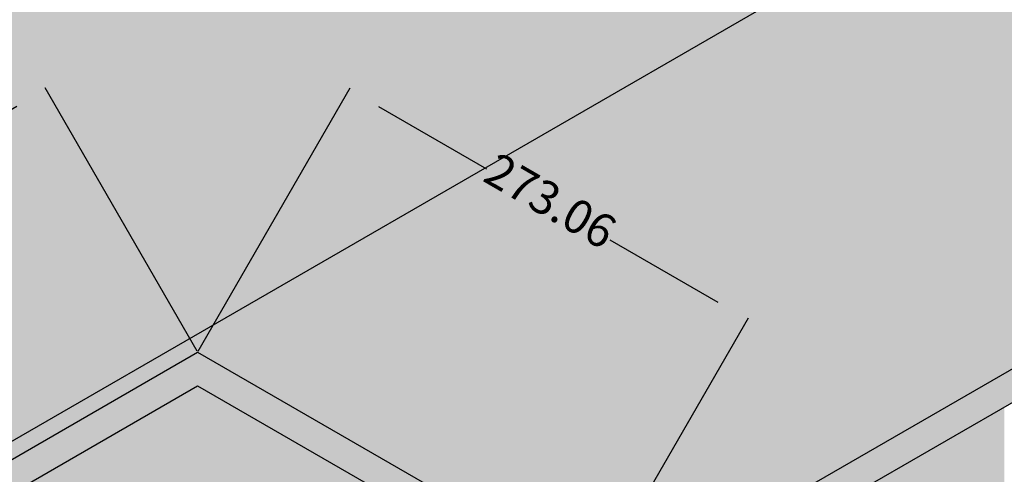
# Model space of a CAD drawing. Units: millimetres. Extents: x 78378 to 86415, y 148682 to 152721.
# Tile 5 of 18: x 79199 to 79783, y 150225 to 150495. Entities that reach past the tile are written whole.
import ezdxf

# ---------------------------------------------------------------- set-up
doc = ezdxf.new("R2010")
doc.units = ezdxf.units.MM
for name, color, linetype, lineweight in [('A-ANNO-DIMS', 2, 'Continuous', 18), ('A-FURN', 4, 'Continuous', 25), ('A-FURN-PATT', 32, 'Continuous', 13)]:
    doc.layers.add(name, color=color, linetype=linetype, lineweight=lineweight)
doc.styles.get("Standard").update_dxf_attribs({"font": 'arial.ttf'})
doc.dimstyles.new('ISO-25', dxfattribs={"dimtxt": 20, "dimasz": 20, "dimexe": 1.25, "dimexo": 0.625, "dimtad": 0, "dimdec": 1, "dimtxsty": 'Standard', "dimcen": 2.5, "dimadec": 0, "dimazin": 0, "dimtfac": 1, "dimtdec": 1, "dimtmove": 0, "dimatfit": 3, "dimfxl": 1, "dimarcsym": 0})

# ---------------------------------------------------------------- blocks, each defined once
blk = doc.blocks.new('*D23')
at = {"layer": 'A-ANNO-DIMS', "color": 0, "lineweight": -2, "transparency": 16777216}
for p, q in [((79304.01, 150298.13), (79213.69, 150454.55)), ((79197, 150443.47), (79082.34, 150377.27)), ((78908.24, 150276.76), (79022.89, 150342.95)), ((78980.6, 150111.41), (78890.29, 150267.84))]:
    blk.add_line(p, q, dxfattribs=at)
at = {"layer": 'A-ANNO-DIMS', "color": 0, "transparency": 16777216}
for points in [[(79195.33, 150446.36), (79198.67, 150440.59), (79214.32, 150453.47)], [(78906.57, 150279.64), (78909.9, 150273.87), (78890.92, 150266.76)]]:
    blk.add_solid(points, dxfattribs=at)
at = {"layer": 'Defpoints', "color": 0, "transparency": 16777216}
for p in [(79214.32, 150453.47), (79304.32, 150297.59), (78980.92, 150110.87)]:
    blk.add_point(p, dxfattribs=at)
at = {"layer": 'A-ANNO-DIMS', "color": 0, "transparency": 16777216, "insert": (79052.62, 150360.11), "char_height": 20, "attachment_point": 5, "rotation": 30}
blk.add_mtext('373.4', dxfattribs=at)
blk = doc.blocks.new('*D24')
at = {"layer": 'A-ANNO-DIMS', "color": 0, "lineweight": -2, "transparency": 16777216}
for p, q in [((79304.63, 150298.13), (79394.94, 150454.55)), ((79411.64, 150443.47), (79475.92, 150406.36)), ((79613.48, 150326.94), (79549.2, 150364.05)), ((79541.11, 150161.6), (79631.43, 150318.02))]:
    blk.add_line(p, q, dxfattribs=at)
at = {"layer": 'A-ANNO-DIMS', "color": 0, "transparency": 16777216}
for points in [[(79413.31, 150446.36), (79409.97, 150440.59), (79394.32, 150453.47)], [(79615.15, 150329.83), (79611.81, 150324.05), (79630.8, 150316.94)]]:
    blk.add_solid(points, dxfattribs=at)
at = {"layer": 'Defpoints', "color": 0, "transparency": 16777216}
for p in [(79630.8, 150316.94), (79304.32, 150297.59), (79540.8, 150161.06)]:
    blk.add_point(p, dxfattribs=at)
at = {"layer": 'A-ANNO-DIMS', "color": 0, "transparency": 16777216, "insert": (79512.56, 150385.21), "char_height": 20, "attachment_point": 5, "rotation": 330}
blk.add_mtext('273.06', dxfattribs=at)

msp = doc.modelspace()

# ---------------------------------------------------------------- hatches: boundary and pattern name
at = {"layer": 'A-FURN-PATT'}
h = msp.add_hatch(color=256, dxfattribs=at)
h.dxf.hatch_style = 1
h.paths.add_polyline_path([(78839.3276, 151040.0076), (78579.52, 151190.0076), (78579.52, 150470.0076), (78839.3276, 150320.0076)])
h.paths.add_polyline_path([(79073.1545, 150899.6469, 0.27777969), (79002.2645, 150996.3205, 0.79108393), (78917.9567, 150978.8719, 0.18044832), (78856.6481, 150853.0138), (78856.6481, 150350.6973), (79073.1545, 150484.318)])
h.paths.add_polyline_path([(79073.1545, 151175.0076), (78856.6481, 151050.0076), (78856.6481, 150853.0138, -0.18044832), (78917.9567, 150978.8719, -0.79108393), (79002.2645, 150996.3205, -0.27777969), (79073.1545, 150899.6469)])
h.paths.add_polyline_path([(79341.6224, 151350.0076), (79099.1352, 151490.0076), (78596.8405, 151200.0076), (78839.3276, 151060.0076)])
h.paths.add_polyline_path([(79904.5389, 151675.0076), (79662.0518, 151815.0076), (79099.1352, 151490.0076), (79341.6224, 151350.0076)])
h.paths.add_polyline_path([(80389.5131, 151955.0076), (80389.5131, 152235.0076), (79662.0518, 151815.0076), (79904.5389, 151675.0076)])
h.paths.add_polyline_path([(80389.5131, 151955.0076), (80164.3465, 151825.0076), (80164.3465, 151105.0076), (80614.6797, 151105.0076), (80614.6797, 151825.0076)])
edge = h.paths.add_edge_path(flags=16)
edge.add_spline(control_points=[(80216.308, 151728.251), (80227.1854, 151732.981), (80256.3301, 151745.6544), (80298.41, 151761.9595), (80340.2597, 151805.855), (80391.0771, 151782.0404), (80454.0396, 151805.7581), (80496.5007, 151742.4095), (80543.8218, 151733.4043), (80562.7182, 151729.8083)], knot_values=[0, 0, 0, 0, 35.54374676, 95.23575347, 136.36767513, 200.93298197, 236.72641081, 322.88993498, 380.17027367, 380.17027367, 380.17027367, 380.17027367], degree=3, periodic=0)
edge.add_line((80562.7182, 151729.8083), (80562.7182, 151165.0076))
edge.add_line((80562.7182, 151165.0076), (80216.308, 151165.0076))
edge.add_line((80216.308, 151165.0076), (80216.308, 151728.251))
h.paths.add_polyline_path([(80632.0002, 152095.0076), (80389.5131, 152235.0076), (80389.5131, 151955.0076), (80614.6797, 151825.0076), (80632.0002, 151815.0076)])
h.paths.add_polyline_path([(80867.7794, 151958.8805), (80632.0002, 152095.0076), (80632.0002, 151815.0076), (80632.0002, 151510.0076), (80867.7794, 151373.8805)])
h.paths.add_polyline_path([(80147.026, 151495.8203, 0.18918979), (80063.5671, 151597.7244, 0.78826136), (79979.2691, 151580.5832, 0.16072613), (79904.5389, 151413.5769), (79904.5389, 150955.0076), (80147.026, 151095.0076)])
h.paths.add_polyline_path([(80147.026, 151815.0076), (79904.5389, 151675.0076), (79904.5389, 151413.5769, -0.16072613), (79979.2691, 151580.5832, -0.78826136), (80063.5671, 151597.7244, -0.18918979), (80147.026, 151495.8203)])
h.paths.add_polyline_path([(79887.2184, 151645.0076), (79640.4011, 151502.5076), (79640.4011, 151262.3325, -0.16072613), (79715.1313, 151429.3387, -0.78826136), (79799.4294, 151446.48, -0.21290578), (79887.2184, 151328.7247)])
h.paths.add_polyline_path([(79799.4294, 151446.48, 0.78826136), (79715.1313, 151429.3387, 0.16072613), (79640.4011, 151262.3325), (79640.4011, 150822.5076), (79887.2184, 150965.0076), (79887.2184, 151328.7247, 0.21290578)])
h.paths.add_polyline_path([(79605.7601, 151482.5076), (79358.9429, 151340.0076), (79358.9429, 151100.0701, -0.16072613), (79433.6731, 151267.0764, -0.78826136), (79517.9711, 151284.2176, -0.21290578), (79605.7601, 151166.4623)])
h.paths.add_polyline_path([(79605.7601, 151166.4623, 0.21290578), (79517.9711, 151284.2176, 0.78826136), (79433.6731, 151267.0764, 0.16072613), (79358.9429, 151100.0701), (79358.9429, 150742.9831), (79419.0877, 150694.7323), (79605.7601, 150802.5076)])
edge = h.paths.add_edge_path(flags=0)
edge.add_spline(control_points=[(81152.4356, 151098.7676), (81105.7208, 151145.9466), (81038.6136, 151213.7208), (80882.3866, 151214.1938), (80797.4434, 151311.2997), (80711.8686, 151340.3754), (80681.7691, 151350.6023)], knot_values=[0, 0, 0, 0, 188.233441, 270.4032752, 445.45179201, 540.42858829, 540.42858829, 540.42858829, 540.42858829], degree=3, periodic=0)
edge.add_line((80683.4538, 151350.0269), (80683.4538, 151104.8792))
edge.add_line((80683.4538, 151104.8792), (81152.4356, 150851.399))
edge.add_line((81152.4356, 150851.399), (81152.4356, 151098.7676))
edge = h.paths.add_edge_path(flags=0)
edge.add_spline(control_points=[(80912.9018, 151027.1103), (80892.3742, 151034.1027), (80860.1663, 151045.0739), (80835.5097, 151068.1214), (80826.5679, 151076.4797)], knot_values=[0, 0, 0, 0, 63.98405104, 100.39142428, 100.39142428, 100.39142428, 100.39142428], degree=3, periodic=0)
edge.add_arc((80830.0414, 151081.2992), 5.9407, 100.9277276, 234.2187381, ccw=False)
edge.add_spline(control_points=[(80828.9152, 151087.1322), (80837.857, 151078.7739), (80862.5136, 151055.7263), (80894.7215, 151044.7552), (80915.2491, 151037.7628)], knot_values=[0, 0, 0, 0, 36.40737324, 100.39142428, 100.39142428, 100.39142428, 100.39142428], degree=3, periodic=0)
edge.add_arc((80914.7882, 151032.2795), 5.5026, -107.9540399, 85.195579, ccw=False)
h.paths.add_polyline_path([(81238.218, 151110.0076), (80632.0002, 151460.0076), (80632.0002, 151105.0076), (81238.218, 150755.0076)])
edge = h.paths.add_edge_path(flags=16)
edge.add_line((81152.4356, 150851.399), (80683.4538, 151104.8792))
edge.add_line((80683.4538, 151104.8792), (80683.4538, 151350.0279))
edge.add_spline(control_points=[(80681.7691, 151350.6023), (80711.8686, 151340.3754), (80797.4434, 151311.2997), (80882.3866, 151214.1938), (81038.6136, 151213.7208), (81105.7208, 151145.9466), (81152.4356, 151098.7676)], knot_values=[0, 0, 0, 0, 94.97679628, 270.02531309, 352.19514729, 540.42858829, 540.42858829, 540.42858829, 540.42858829], degree=3, periodic=0)
edge.add_line((81152.4356, 151098.7676), (81152.4356, 150851.399))
edge = h.paths.add_edge_path(flags=0)
edge.add_spline(control_points=[(80912.9018, 151027.1103), (80892.3742, 151034.1027), (80860.1663, 151045.0739), (80835.5097, 151068.1214), (80826.5679, 151076.4797)], knot_values=[0, 0, 0, 0, 63.98405104, 100.39142428, 100.39142428, 100.39142428, 100.39142428], degree=3, periodic=0)
edge.add_arc((80830.0414, 151081.2992), 5.9407, 100.9277276, 234.2187381, ccw=False)
edge.add_spline(control_points=[(80828.9152, 151087.1322), (80837.857, 151078.7739), (80862.5136, 151055.7263), (80894.7215, 151044.7552), (80915.2491, 151037.7628)], knot_values=[0, 0, 0, 0, 36.40737324, 100.39142428, 100.39142428, 100.39142428, 100.39142428], degree=3, periodic=0)
edge.add_arc((80914.7882, 151032.2795), 5.5026, -107.7417882, 85.195579, ccw=False)
h.paths.add_polyline_path([(81498.0256, 151255.0076), (81238.218, 151110.0076), (81238.218, 150755.0076), (81498.0256, 150905.0076)])
edge = h.paths.add_edge_path(flags=16)
edge.add_spline(control_points=[(81152.4356, 151098.7676), (81105.7208, 151145.9466), (81038.6136, 151213.7208), (80882.3866, 151214.1938), (80797.4434, 151311.2997), (80711.8686, 151340.3754), (80681.7691, 151350.6023)], knot_values=[0, 0, 0, 0, 188.233441, 270.4032752, 445.45179201, 540.42858829, 540.42858829, 540.42858829, 540.42858829], degree=3, periodic=0)
edge.add_line((80683.4538, 151350.0279), (80683.4538, 151104.8792))
edge.add_line((80683.4538, 151104.8792), (81152.4356, 150851.399))
edge.add_line((81152.4356, 150851.399), (81152.4356, 151098.7676))
h.paths.add_polyline_path([(81453.9904, 151280.4314), (80867.7794, 151618.8805), (80867.7794, 151373.8805), (81238.218, 151160.0076)])
edge = h.paths.add_edge_path(flags=16)
edge.add_line((81189.2304, 151297.6373), (81114.4166, 151300.2154))
edge.add_arc((81412.0967, 151394.0167), 312.1092, 179.7569303, 197.4900342, ccw=False)
edge.add_ellipse((81154.0183, 151392.0436), major_axis=(-54.0264, 3.6301), ratio=0.22179693, start_angle=0, end_angle=0.3517985, ccw=False)
edge.add_ellipse((81154.0183, 151392.0436), major_axis=(-54.0264, 3.6301), ratio=0.22179693, start_angle=180, end_angle=360, ccw=False)
edge.add_spline(control_points=[(81196.1844, 151321.9476), (81224.9802, 151347.1455), (81266.8846, 151383.8144), (81222.0354, 151387.0304), (81208.0056, 151388.0364)], knot_values=[0, 0, 0, 0, 75.09175173, 109.27580439, 109.27580439, 109.27580439, 109.27580439], degree=3, periodic=0)
edge.add_arc((80751.9112, 151435.6145), 458.5693, 342.4891602, 345.646172, ccw=False)
edge = h.paths.add_edge_path(flags=0)
edge.add_spline(control_points=[(81196.6193, 151323.657), (81197.893, 151324.7717), (81199.1654, 151325.8858), (81209.0233, 151334.5343), (81217.3959, 151341.9835), (81228.0928, 151352.5012), (81231.3883, 151355.9524), (81236.9493, 151362.4395), (81239.214, 151365.4773), (81241.4987, 151369.416), (81242.064, 151370.5542), (81242.9187, 151372.6971), (81243.2076, 151373.7015), (81243.5012, 151375.5539), (81243.5065, 151376.4), (81243.2432, 151377.9407), (81242.9775, 151378.6373), (81242.1402, 151379.937), (81241.5659, 151380.5416), (81240.2039, 151381.533), (81239.4963, 151381.9384), (81237.0619, 151383.0663), (81235.0242, 151383.6999), (81230.352, 151384.7569), (81227.7173, 151385.1826), (81221.9118, 151385.9145), (81218.7193, 151386.2133), (81213.7912, 151386.6115), (81212.1252, 151386.7359), (81209.6196, 151386.9181), (81208.7865, 151386.9779), (81207.9009, 151387.0432)], knot_values=[0.01548744, 0.01548744, 0.01548744, 0.01548744, 3.33787957, 3.33787957, 25.85130624, 25.85130624, 37.52811308, 37.52811308, 49.20491992, 49.20491992, 54.2850938, 54.2850938, 59.36526768, 59.36526768, 64.44544157, 64.44544157, 69.52561545, 69.52561545, 74.60578933, 74.60578933, 78.49366785, 78.49366785, 86.25567095, 86.25567095, 94.01767406, 94.01767406, 102.20226556, 102.20226556, 106.29456131, 106.29456131, 108.32522175, 108.32522175, 108.32522175, 108.32522175], degree=3, periodic=0)
edge = h.paths.add_edge_path(flags=16)
edge.add_arc((81034.1732, 151350.4693), 42.5822, 231.2679035, 306.151846, ccw=False)
edge.add_line((81007.5303, 151317.2517), (81007.5303, 151395.181))
edge.add_ellipse((81033.412, 151394.7791), major_axis=(-25.8816, 0.4538), ratio=0.23894509, start_angle=0, end_angle=0.1147075, ccw=False)
edge.add_ellipse((81033.412, 151394.7791), major_axis=(-25.8816, 0.4538), ratio=0.23894509, start_angle=181.1677709, end_angle=358.9476457, ccw=False)
edge.add_ellipse((81033.412, 151395.7791), major_axis=(-25.8816, 0.4538), ratio=0.23894509, start_angle=180, end_angle=360.1147075, ccw=False)
edge.add_ellipse((81033.412, 151395.7791), major_axis=(-25.8816, 0.4538), ratio=0.23894509, start_angle=178.9476457, end_angle=180, ccw=False)
edge.add_line((81059.2936, 151395.1778), (81059.2936, 151394.3772))
edge.add_ellipse((81033.412, 151394.7791), major_axis=(-25.8816, 0.4538), ratio=0.23894509, start_angle=180, end_angle=180.1147075, ccw=False)
edge.add_ellipse((81033.412, 151394.7791), major_axis=(-25.8816, 0.4538), ratio=0.23894509, start_angle=3.6903098, end_angle=176.4406503, ccw=False)
edge.add_line((81059.2936, 151393.3388), (81059.2936, 151316.086))
h.paths.add_polyline_path([(80951.9355, 151343.9568), (80909.6838, 151362.4635), (80904.0219, 151443.9615, -0.38133308), (80987.2169, 151411.3717)], flags=16)
h = msp.add_hatch(color=256, dxfattribs=at)
h.dxf.hatch_style = 1
h.paths.add_polyline_path([(80389.8136, 150935.1811), (80389.5131, 151105.0076), (80164.3465, 151105.0076), (79904.5389, 150955.0076), (79433.5848, 150683.1022), (79459.4128, 150662.3818), (79243.9048, 150537.9582), (79160.4069, 150518.1674), (78839.3276, 150320.0076), (78579.52, 150470.0076), (78570.8597, 150475.0076), (78570.8597, 150465.0076), (78570.8597, 149885.0076)])
h.paths.add_polyline_path([(80086.4042, 150460.0076), (79826.5966, 150610.0076), (78570.8597, 149885.0076), (78830.6674, 149735.0076)])
h.paths.add_polyline_path([(79540.8001, 150161.0557), (79217.3967, 149974.3386), (78980.9166, 150110.8705), (79304.32, 150297.5875)], flags=16)
h.paths.add_polyline_path([(79506.159, 150161.0557), (79217.3967, 149994.3386), (79015.5576, 150110.8705), (79304.32, 150277.5875)], flags=0)
edge = h.paths.add_edge_path(flags=0)
edge.add_arc((79247.8636, 150177.1541), 137.9799, 256.0025928, 293.5594109)
edge.add_arc((79240.7671, 150078.2605), 68.0855, 336.099104, 387.3696877)
edge.add_ellipse((79258.3074, 150109.4852), major_axis=(-42.6234, -1.6591), ratio=0.16042843, start_angle=0, end_angle=179.0977279, ccw=False)
edge.add_arc((79285.2112, 150074.2509), 77.2096, 155.1233104, 203.6557939)
edge = h.paths.add_edge_path(flags=0)
edge.add_ellipse((79258.6958, 150110.8297), major_axis=(-42.6234, -1.6591), ratio=0.16042843, start_angle=350.6039412, end_angle=356.2289762)
edge.add_line((79219.169, 150111.8937), (79218.3268, 150109.4141))
edge.add_arc((79262.4675, 150032.9602), 88.2813, 112.3931229, 120, ccw=False)
h.paths.add_polyline_path([(79287.0625, 150086.9703, -0.24770206), (79288.1967, 150077.2955, -0.39047651), (79265.4731, 150072.5438, -0.48726153), (79264.079, 150082.3769, 0.39560433)], flags=0)
h.paths.add_polyline_path([(80389.5131, 150935.0076), (79826.5966, 150610.0076), (80086.4042, 150460.0076), (80692.622, 150460.0076), (80952.4296, 150610.0076)])
edge = h.paths.add_edge_path(flags=16)
edge.add_ellipse((80392.4466, 150825.601), major_axis=(-133.0757, 7.722), ratio=0.42449957, start_angle=0, end_angle=360)
edge = h.paths.add_edge_path(flags=0)
edge.add_spline(control_points=[(80269.3541, 150832.7436), (80269.2919, 150831.672), (80269.3503, 150830.5922), (80269.7341, 150828.3361), (80270.0612, 150827.1587), (80271.0461, 150824.6748), (80271.7052, 150823.3692), (80273.4061, 150820.6503), (80274.4481, 150819.2381), (80276.9366, 150816.3509), (80278.3828, 150814.8762), (80282.5858, 150811.0913), (80285.6261, 150808.7701), (80292.6031, 150804.2267), (80296.5388, 150802.0041), (80305.195, 150797.7581), (80309.9151, 150795.7344), (80320.0112, 150791.96), (80325.387, 150790.2092), (80339.2162, 150786.315), (80347.9578, 150784.3563), (80366.0679, 150781.2568), (80375.4359, 150780.1158), (80394.3093, 150778.7158), (80403.8142, 150778.4568), (80422.4656, 150778.8319), (80431.6115, 150779.4662), (80449.0608, 150781.5838), (80457.3636, 150783.0675), (80472.6699, 150786.7766), (80479.6726, 150789.0033), (80490.1894, 150793.2813), (80494.1268, 150795.1967), (80501.0146, 150799.1885), (80503.9632, 150801.2651), (80508.2066, 150804.9015), (80509.73, 150806.4609), (80512.1996, 150809.4942), (80513.1456, 150810.9657), (80514.4291, 150813.5431), (80514.8436, 150814.6688), (80515.3984, 150816.8625), (80515.5405, 150817.9315), (80515.5801, 150820.098), (80515.4773, 150821.1978), (80514.9905, 150823.5062), (80514.6047, 150824.7154), (80513.4854, 150827.2641), (80512.7511, 150828.6027), (80510.8872, 150831.3809), (80509.7578, 150832.8196), (80507.0873, 150835.7513), (80505.5466, 150837.2439), (80501.0624, 150841.0944), (80497.8199, 150843.4576), (80490.4174, 150848.062), (80486.2582, 150850.3037), (80477.1448, 150854.5643), (80472.1909, 150856.5835), (80461.6275, 150860.3245), (80456.0182, 150862.0465), (80441.7332, 150865.8127), (80432.7885, 150867.6675), (80414.3391, 150870.5317), (80404.8349, 150871.5411), (80385.7707, 150872.6572), (80376.2113, 150872.764), (80357.5444, 150872.0728), (80348.4375, 150871.2748), (80331.1682, 150868.83), (80323.0064, 150867.1827), (80309.472, 150863.5363), (80303.8628, 150861.6593), (80293.8018, 150857.5401), (80289.3512, 150855.2969), (80282.7757, 150851.2345), (80280.3473, 150849.4579), (80276.2606, 150845.9127), (80274.604, 150844.1458), (80272.3157, 150841.1243), (80271.5358, 150839.8454), (80270.3496, 150837.3879), (80269.9417, 150836.2101), (80269.5065, 150834.2815), (80269.3988, 150833.5143), (80269.3541, 150832.7436)], knot_values=[0, 0, 0, 0, 0.09750046, 0.09750046, 0.19500092, 0.19500092, 0.29250138, 0.29250138, 0.39000184, 0.39000184, 0.4875023, 0.4875023, 0.63880322, 0.63880322, 0.79010415, 0.79010415, 0.94140507, 0.94140507, 1.092706, 1.092706, 1.3128171, 1.3128171, 1.5329282, 1.5329282, 1.7530393, 1.7530393, 1.97315041, 1.97315041, 2.19326151, 2.19326151, 2.41337261, 2.41337261, 2.56986063, 2.56986063, 2.72634866, 2.72634866, 2.84418658, 2.84418658, 2.96202451, 2.96202451, 3.06023388, 3.06023388, 3.15844325, 3.15844325, 3.25665261, 3.25665261, 3.35486198, 3.35486198, 3.45307135, 3.45307135, 3.55128072, 3.55128072, 3.64949009, 3.64949009, 3.80392773, 3.80392773, 3.95836537, 3.95836537, 4.11280301, 4.11280301, 4.26724064, 4.26724064, 4.48920349, 4.48920349, 4.71116635, 4.71116635, 4.9331292, 4.9331292, 5.15509205, 5.15509205, 5.3770549, 5.3770549, 5.55785361, 5.55785361, 5.73865232, 5.73865232, 5.87239556, 5.87239556, 6.00613879, 6.00613879, 6.109605, 6.109605, 6.2130712, 6.2130712, 6.28318531, 6.28318531, 6.28318531, 6.28318531], degree=3, periodic=0)
edge = h.paths.add_edge_path(flags=0)
edge.add_ellipse((80392.4466, 150825.601), major_axis=(-101.8398, 3.3923), ratio=0.40349248, start_angle=0, end_angle=360)
edge = h.paths.add_edge_path(flags=0)
edge.add_ellipse((80391.1657, 150858.3746), major_axis=(9.0882, -0.6733), ratio=0.35135413, start_angle=0, end_angle=360)
h.paths.add_polyline_path([(80952.4296, 150610.0076), (80692.622, 150460.0076), (81361.2342, 150073.9842), (81649.9628, 150052.7286), (81766.4935, 150120.0076), (81766.4935, 150140.0076), (81564.9025, 150256.3963), (81564.8884, 150096.1963), (81538.9076, 150111.1963), (81538.9217, 150271.3963)])
h.paths.add_polyline_path([(81539.0357, 151571.3305), (80867.7794, 151958.8805), (80867.7794, 151618.8805), (81498.0256, 151255.0076), (81498.0256, 150905.0076), (81238.218, 150755.0076), (81538.9488, 150581.3806)])
h.paths.add_polyline_path([(81766.4935, 151440.0076), (81565.0164, 151556.3305), (81564.9296, 150566.3806), (81766.4935, 150450.0076)])
edge = h.paths.add_edge_path()
edge.add_line((81564.9296, 150566.3806), (81564.9137, 150384.6289))
edge.add_ellipse((81552.1304, 150358.5718), major_axis=(52.6272, 3.506), ratio=0.49589905, start_angle=367.5169757, end_angle=420.0564686, ccw=False)
edge.add_ellipse((81552.1304, 150358.5718), major_axis=(52.6272, 3.506), ratio=0.49589905, start_angle=351.729742, end_angle=367.5169757, ccw=False)
edge.add_ellipse((81552.1304, 150345.5016), major_axis=(52.6272, 3.506), ratio=0.49589905, start_angle=352.5116949, end_angle=366.3006092, ccw=False)
edge.add_line((81603.4463, 150342.2039), (81603.5064, 150340.4475))
edge.add_ellipse((81552.1304, 150332.128), major_axis=(52.6272, 3.506), ratio=0.49589905, start_angle=353.6729654, end_angle=365.3867997, ccw=False)
edge.add_ellipse((81552.1304, 150332.128), major_axis=(52.6272, 3.506), ratio=0.49589905, start_angle=350.9388331, end_angle=353.6729654)
edge.add_line((81603.8688, 150329.855), (81604.0442, 150324.7302))
edge.add_ellipse((81552.1304, 150317.7418), major_axis=(52.6272, 3.506), ratio=0.49589905, start_angle=355.2176746, end_angle=363.8553364, ccw=False)
edge.add_ellipse((81552.1304, 150317.7418), major_axis=(52.6272, 3.506), ratio=0.49589905, start_angle=341.3250873, end_angle=355.2176746, ccw=False)
edge.add_ellipse((81552.1304, 150317.7418), major_axis=(52.6272, 3.506), ratio=0.49589905, start_angle=293.4661701, end_angle=341.3250873, ccw=False)
edge.add_line((81564.9057, 150292.9664), (81564.9025, 150256.3963))
edge.add_line((81564.9025, 150256.3963), (81766.4935, 150140.0076))
edge.add_line((81766.4935, 150140.0076), (81766.4935, 150450.0076))
edge.add_line((81766.4935, 150450.0076), (81564.9296, 150566.3806))
h.paths.add_polyline_path([(81525.5713, 150321.598), (81526.5985, 150321.3069), (81528.6771, 150320.947)])
h.paths.add_polyline_path([(81512.7903, 150326.1129), (81514.5058, 150325.3887), (81512.538, 150326.2678)])
h.paths.add_polyline_path([(81533.2148, 150320.1615), (81534.6952, 150319.9052), (81536.5995, 150319.7557)])
h.paths.add_polyline_path([(81518.622, 150323.6513), (81519.227, 150323.3959), (81521.289, 150322.8116)])
h.paths.add_polyline_path([(81501.2183, 150336.2599), (81500.3543, 150338.1339), (81499.7815, 150340.0494), (81499.5032, 150341.9955), (81499.5032, 150343.7257), (81499.7584, 150345.5905), (81500.2766, 150347.4549), (81501.0551, 150349.3095), (81501.0967, 150349.3937), (81501.1389, 150349.4778), (81500.9978, 150349.7496), (81500.8628, 150350.0225), (81499.5032, 150355.0658), (81499.9591, 150359.5002), (81501.8982, 150363.9083), (81505.2653, 150368.1646), (81509.9647, 150372.1482), (81515.8627, 150375.7459), (81522.7918, 150378.8553), (81530.555, 150381.3882), (81538.9315, 150383.2724), (81538.9488, 150581.3806), (80632.0002, 151105.0076), (80389.5131, 151105.0076), (80389.8142, 150934.8338), (80952.4296, 150610.0076), (81538.9217, 150271.3963), (81538.9234, 150291.7194), (81538.8752, 150291.721), (81530.1915, 150292.8239), (81522.1802, 150294.6904), (81515.0866, 150297.2633), (81509.8635, 150299.9959), (81505.6084, 150303.1351), (81502.419, 150306.6088), (81500.3683, 150310.3375), (81499.5032, 150314.2358), (81499.5032, 150315.9659), (81499.8206, 150318.1159), (81500.487, 150320.2634), (81501.4979, 150322.3941), (81500.487, 150324.4233), (81499.8206, 150326.5039), (81499.5032, 150328.622), (81499.5032, 150330.3521), (81499.7815, 150332.3262), (81500.3543, 150334.2992)])
h = msp.add_hatch(color=256, dxfattribs=at)
h.dxf.hatch_style = 1
h.paths.add_polyline_path([(79090.475, 151205.0076), (78839.3276, 151060.0076), (78839.3276, 150320.0076), (79090.475, 150475.0076)])
h.paths.add_polyline_path([(79073.1545, 151175.0076), (79073.1545, 150899.6469, -0.04544363), (79073.1545, 150878.5653), (79073.1545, 150484.318), (78856.6481, 150350.6973), (78856.6481, 150814.5249, -0.04815716), (78856.6481, 150853.0138), (78856.6481, 151050.0076)], flags=16)
h.paths.add_polyline_path([(79358.9429, 151340.0076), (79605.7601, 151482.5076), (79605.7601, 150802.5076), (79419.0877, 150694.7323), (79433.5848, 150683.1022), (79623.0806, 150792.5076), (79623.0806, 151512.5076), (79341.6224, 151350.0076), (79341.6224, 150756.8784), (79358.9429, 150742.9831)])
h.paths.add_polyline_path([(79341.6224, 151350.0076), (79090.475, 151205.0076), (79090.475, 150475.0076), (79160.4069, 150518.1674), (79107.7955, 150505.6973), (79107.7955, 151195.0076), (79109.5275, 151196.0076), (79324.3018, 151320.0076), (79324.3018, 150770.7736), (79341.6224, 150756.8784)])
h.paths.add_polyline_path([(79887.2184, 151645.0076), (79887.2184, 151665.0076), (79623.0806, 151512.5076), (79623.0806, 150792.5076), (79887.2184, 150945.0076), (79887.2184, 150965.0076), (79640.4011, 150822.5076), (79640.4011, 151502.5076)])
h.paths.add_polyline_path([(79904.5389, 151655.0076), (79887.2184, 151645.0076), (79887.2184, 150965.0076), (79904.5389, 150975.0076)])
h.paths.add_polyline_path([(80164.3465, 151825.0076), (80147.026, 151815.0076), (80147.026, 151095.0076), (80164.3465, 151105.0076)])
h.paths.add_polyline_path([(80632.0002, 151510.0076), (80632.0002, 151490.0076), (81238.218, 151140.0076), (81471.6045, 151270.2619), (81453.9904, 151280.4314), (81238.218, 151160.0076)])
h.paths.add_polyline_path([(80632.0002, 151490.0076), (80632.0002, 151470.0076), (81238.218, 151120.0076), (81489.2186, 151260.0924), (81471.6045, 151270.2619), (81238.218, 151140.0076)])
h.paths.add_polyline_path([(80632.0002, 151460.0076), (80632.0002, 151105.0076), (81238.218, 150755.0076), (81238.218, 151110.0076)])
edge = h.paths.add_edge_path(flags=16)
edge.add_spline(control_points=[(80681.7691, 151350.6023), (80711.8686, 151340.3754), (80797.4434, 151311.2997), (80882.3866, 151214.1938), (81038.6136, 151213.7208), (81105.7208, 151145.9466), (81152.4356, 151098.7676)], knot_values=[0, 0, 0, 0, 94.97679628, 270.02531309, 352.19514729, 540.42858829, 540.42858829, 540.42858829, 540.42858829], degree=3, periodic=0)
edge.add_line((81152.4356, 151098.7676), (81152.4356, 150851.399))
edge.add_line((81152.4356, 150851.399), (80683.4538, 151104.8792))
edge.add_line((80683.4538, 151104.8792), (80683.4538, 151350.027))
edge = h.paths.add_edge_path(flags=0)
edge.add_spline(control_points=[(80828.9152, 151087.1322), (80837.857, 151078.7739), (80862.5136, 151055.7263), (80894.7215, 151044.7552), (80915.2491, 151037.7628)], knot_values=[0, 0, 0, 0, 36.40737324, 100.39142428, 100.39142428, 100.39142428, 100.39142428], degree=3, periodic=0)
edge.add_arc((80914.7882, 151032.2795), 5.5026, -107.9540399, 85.195579, ccw=False)
edge.add_spline(control_points=[(80912.9018, 151027.1103), (80892.3742, 151034.1027), (80860.1663, 151045.0739), (80835.5097, 151068.1214), (80826.5679, 151076.4797)], knot_values=[0, 0, 0, 0, 63.98405104, 100.39142428, 100.39142428, 100.39142428, 100.39142428], degree=3, periodic=0)
edge.add_arc((80830.0414, 151081.2992), 5.9407, 100.9277276, 234.2187381, ccw=False)
h.paths.add_polyline_path([(80632.0002, 151815.0076), (80614.6797, 151825.0076), (80614.6797, 151105.0076), (80632.0002, 151105.0076)])
h.paths.add_polyline_path([(81498.0256, 151255.0076), (81489.2186, 151260.0924), (81238.218, 151120.0076), (80632.0002, 151470.0076), (80632.0002, 151460.0076), (81238.218, 151110.0076)])
h.paths.add_polyline_path([(78596.8405, 151200.0076), (78579.52, 151190.0076), (78839.3276, 151040.0076), (78839.3276, 151060.0076)])
h.paths.add_polyline_path([(78596.8405, 151200.0076), (78579.52, 151210.0076), (78579.52, 151190.0076)])
h.paths.add_polyline_path([(78579.52, 151210.0076), (78570.8597, 151205.0076), (78570.8597, 150475.0076), (78579.52, 150470.0076)])
h = msp.add_hatch(color=256, dxfattribs=at)
h.dxf.hatch_style = 1
h.paths.add_polyline_path([(79783.2953, 150265.0076), (79783.2953, 150285.0076), (79257.8556, 149981.6449), (79257.8556, 149961.6449)])
h.paths.add_polyline_path([(80086.4042, 150440.0076), (80086.4042, 150460.0076), (79783.2953, 150285.0076), (79783.2953, 150265.0076)])
h = msp.add_hatch(color=256, dxfattribs=at)
h.dxf.hatch_style = 1
h.paths.add_polyline_path([(79304.32, 150297.5875), (78980.9166, 150110.8705), (79217.3967, 149974.3386), (79540.8001, 150161.0557)])
h.paths.add_polyline_path([(79506.159, 150161.0557), (79217.3967, 149994.3386), (79015.5576, 150110.8705), (79304.32, 150277.5875)], flags=16)
edge = h.paths.add_edge_path(flags=0)
edge.add_line((79260.8583, 150135.9631), (79296.366, 150115.4627))
edge.add_ellipse((79258.6958, 150110.8297), major_axis=(-42.6234, -1.6591), ratio=0.16042843, start_angle=540.1624997, end_angle=544.7822411, ccw=False)
edge.add_ellipse((79258.6958, 150110.8297), major_axis=(-42.6234, -1.6591), ratio=0.16042843, start_angle=540, end_angle=540.1624997, ccw=False)
edge.add_line((79301.3113, 150112.6075), (79301.4117, 150112.5496))
edge.add_ellipse((79258.6958, 150110.8297), major_axis=(-42.6234, -1.6591), ratio=0.16042843, start_angle=538.60644, end_angle=539.6688473, ccw=False)
edge.add_arc((79299.1378, 150112.0107), 2.2333, -43.6788662, 8.9937503, ccw=False)
edge.add_arc((79240.7671, 150078.2605), 68.0855, -23.900896, 28.2323958, ccw=False)
edge.add_arc((79247.8636, 150177.1541), 137.9799, 256.0025928, 293.5594109, ccw=False)
edge.add_arc((79285.2112, 150074.2509), 77.2096, 154.2238314, 203.6557939, ccw=False)
edge.add_ellipse((79258.3074, 150109.4852), major_axis=(-42.6234, -1.6591), ratio=0.16042843, start_angle=359.9882645, end_angle=360, ccw=False)
edge.add_arc((79216.8461, 150108.3941), 1.2901, 125.5884183, 205.6940851, ccw=False)
edge.add_ellipse((79258.6958, 150110.8297), major_axis=(-42.6234, -1.6591), ratio=0.16042843, start_angle=358.1218837, end_angle=359.634987, ccw=False)
edge.add_line((79216.51, 150110.3586), (79216.8824, 150110.5736))
edge.add_ellipse((79258.6958, 150110.8297), major_axis=(-42.6234, -1.6591), ratio=0.16042843, start_angle=356.2289762, end_angle=358.1218837, ccw=False)
edge.add_line((79219.169, 150111.8937), (79260.8583, 150135.9631))
h.paths.add_polyline_path([(79288.1967, 150077.2955, -0.39047651), (79265.4731, 150072.5438, -0.48726153), (79264.079, 150082.3769, 0.39560433), (79287.0625, 150086.9703, -0.24770206)], flags=0)
h = msp.add_hatch(color=256, dxfattribs=at)
h.dxf.hatch_style = 1
edge = h.paths.add_edge_path()
edge.add_line((79506.159, 150161.0557), (79405.2395, 150219.3216))
edge.add_line((79405.2395, 150219.3216), (79260.8583, 150135.9631))
edge.add_line((79260.8583, 150135.9631), (79296.366, 150115.4627))
edge.add_ellipse((79258.6958, 150110.8297), major_axis=(-42.6234, -1.6591), ratio=0.16042843, start_angle=540.1624997, end_angle=544.7822411, ccw=False)
edge.add_ellipse((79258.6958, 150110.8297), major_axis=(-42.6234, -1.6591), ratio=0.16042843, start_angle=538.60644, end_angle=539.6688473, ccw=False)
edge.add_line((79301.4117, 150112.5496), (79361.7779, 150077.6971))
edge.add_line((79361.7779, 150077.6971), (79506.159, 150161.0557))
h.paths.add_polyline_path([(79405.2395, 150219.3216), (79304.32, 150277.5875), (79159.9388, 150194.229), (79260.8583, 150135.9631)])
edge = h.paths.add_edge_path()
edge.add_line((79260.8583, 150135.9631), (79159.9388, 150194.229))
edge.add_line((79159.9388, 150194.229), (79015.5576, 150110.8705))
edge.add_line((79015.5576, 150110.8705), (79116.4771, 150052.6045))
edge.add_line((79116.4771, 150052.6045), (79216.8824, 150110.5736))
edge.add_ellipse((79258.6958, 150110.8297), major_axis=(-42.6234, -1.6591), ratio=0.16042843, start_angle=356.2289762, end_angle=358.1218837, ccw=False)
edge.add_ellipse((79258.6958, 150110.8297), major_axis=(-42.6234, -1.6591), ratio=0.16042843, start_angle=350.6039412, end_angle=356.2289762)
edge.add_line((79219.169, 150111.8937), (79260.8583, 150135.9631))
h.paths.add_polyline_path([(79300.7529, 150110.4683, 0.21642229), (79301.362, 150112.2118, 0.25927743), (79215.6839, 150107.826, 0.21909574), (79214.4893, 150043.2712, 0.16535535), (79303.0141, 150050.6753, 0.23148087)], flags=16)
h.paths.add_polyline_path([(79264.079, 150082.3769, 0.39560433), (79287.0625, 150086.9703, -0.24770206), (79288.1967, 150077.2955, -0.39047651), (79265.4731, 150072.5438, -0.48726153)], flags=0)
h.paths.add_polyline_path([(79361.7779, 150077.6971), (79301.4117, 150112.5496), (79260.8583, 150135.9631), (79116.4771, 150052.6045), (79217.3967, 149994.3386)])
edge = h.paths.add_edge_path(flags=16)
edge.add_ellipse((79258.3074, 150109.4852), major_axis=(-42.6234, -1.6591), ratio=0.16042843, start_angle=180.4067093, end_angle=238.2058938, ccw=False)
edge.add_arc((79299.1378, 150112.0107), 2.2333, 335.7071144, 365.168126)
edge.add_arc((79262.4675, 150032.9602), 88.2813, 63.8595099, 90.1998686)
edge.add_arc((79256.9649, 150118.7368), 5.7667, -23.3220096, 25.7370753, ccw=False)
edge = h.paths.add_edge_path(flags=0)
edge.add_ellipse((79258.3074, 150109.4852), major_axis=(-42.6234, -1.6591), ratio=0.16042843, start_angle=0, end_angle=179.0977279, ccw=False)
edge.add_arc((79285.2112, 150074.2509), 77.2096, 154.2238314, 203.6557939)
edge.add_arc((79247.8636, 150177.1541), 137.9799, 256.0025928, 293.5594109)
edge.add_arc((79240.7671, 150078.2605), 68.0855, 336.099104, 388.2323958)
h = msp.add_hatch(color=256, dxfattribs=at)
h.dxf.hatch_style = 1
h.paths.add_polyline_path([(79765.9748, 150214.3024), (79275.1761, 149930.9396), (79275.1761, 149340.2556), (79361.1019, 149389.8649), (79361.1019, 149854.0252), (79688.5392, 150043.0712), (79688.5392, 149578.9109), (79765.9748, 149623.6184)], flags=0)
h.paths.add_polyline_path([(79616.9975, 150064.3358, -1), (79579.5778, 150064.3358, -1)], flags=0)
h.paths.add_polyline_path([(79511.257, 150003.2865, -1), (79473.8373, 150003.2865, -1)], flags=0)
h.paths.add_polyline_path([(79398.6146, 149938.2524, -1), (79361.1949, 149938.2524, -1)], flags=0)
h.paths.add_polyline_path([(79688.5392, 149578.9109), (79667.1607, 149674.8368), (79401.2524, 149521.3146), (79361.1019, 149389.8649)], flags=0)
h.paths.add_polyline_path([(79783.2953, 149613.6184), (79783.2953, 150126.6366), (79783.2953, 150265.0076), (79257.8556, 149961.6449), (79257.8556, 149310.2556)])
h.paths.add_polyline_path([(79275.1761, 149340.2556), (79275.1761, 149930.9396), (79765.9748, 150214.3024), (79765.9748, 149623.6184)], flags=16)
h.paths.add_polyline_path([(79361.1019, 149389.8649), (79361.1019, 149854.0252), (79688.5392, 150043.0712), (79688.5392, 149578.9109), (79667.1607, 149674.8368), (79401.2524, 149521.3146)], flags=0)
h.paths.add_polyline_path([(79477.9029, 149864.6773), (79477.9029, 149877.6076), (79571.7852, 149931.8105), (79571.7852, 149918.8803)], flags=0)

# ---------------------------------------------------------------- linework, layer by layer
at = {"layer": 'A-FURN'}
for p, q in [((78570.8597, 149885.0076), (80389.5131, 150935.0076)), ((78830.6674, 149735.0076), (80086.4042, 150460.0076)), ((79257.8556, 149961.6449), (80086.4042, 150440.0076)), ((78980.9166, 150110.8705), (79304.32, 150297.5875)), ((79304.32, 150297.5875), (79540.8001, 150161.0557)), ((79015.5576, 150110.8705), (79304.32, 150277.5875)), ((79304.32, 150277.5875), (79506.159, 150161.0557))]:
    msp.add_line(p, q, dxfattribs=at)

# ---------------------------------------------------------------- dimensions: what is measured, and where the dimension line sits
at = {"layer": 'A-ANNO-DIMS'}
for base, p1, p2, angle, override, picture, middle in [((79214.32, 150453.4721), (78980.9166, 150110.8705), (79304.32, 150297.5875), 30, {"dimdec": 1, "dimlfac": 1, "dimrnd": 0, "dimzin": 0, "dimdsep": 46, "dimlunit": 2}, '*D23', (79052.6183, 150360.1136)), ((79630.8001, 150316.9402), (79304.32, 150297.5875), (79540.8001, 150161.0557), 330, {"dimdec": 2, "dimlfac": 1, "dimrnd": 0, "dimzin": 0, "dimdsep": 46, "dimlunit": 2}, '*D24', (79512.56, 150385.2062))]:
    dim = msp.add_linear_dim(base=base, p1=p1, p2=p2, angle=angle, dimstyle='ISO-25', override=override, dxfattribs=at)
    dim.commit()
    dim.dimension.update_dxf_attribs({"geometry": picture, "text_midpoint": middle})

doc.saveas('drawing.dxf')
